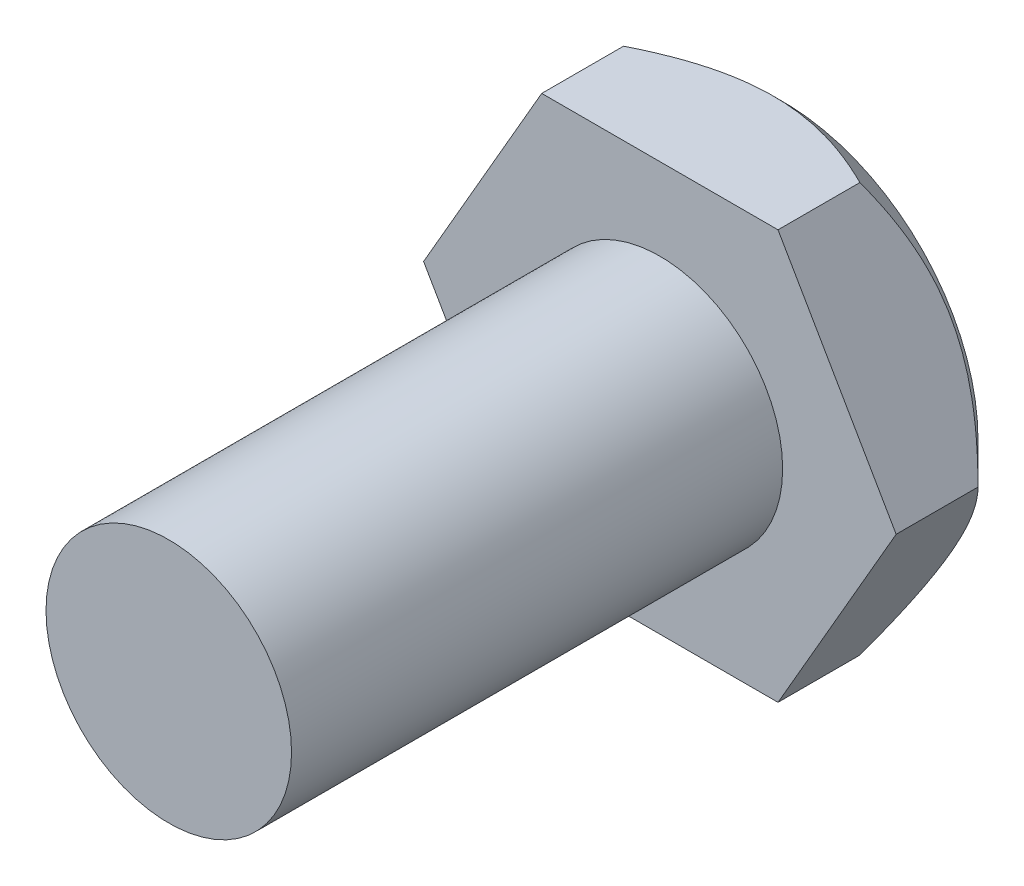
ISO-10303-21;
HEADER;
FILE_DESCRIPTION(('STEP AP214'),'2;1');
FILE_NAME('part.step','',(''),(''),'','','');
FILE_SCHEMA(('AUTOMOTIVE_DESIGN { 1 0 10303 214 1 1 1 1 }'));
ENDSEC;
DATA;
#1=APPLICATION_CONTEXT('core data for automotive mechanical design processes');
#2=APPLICATION_PROTOCOL_DEFINITION('international standard','automotive_design',2000,#1);
#3=PRODUCT_CONTEXT('',#1,'mechanical');
#4=PRODUCT('Part','Part','',(#3));
#5=PRODUCT_RELATED_PRODUCT_CATEGORY('part','',(#4));
#6=PRODUCT_DEFINITION_FORMATION('','',#4);
#7=PRODUCT_DEFINITION_CONTEXT('part definition',#1,'design');
#8=PRODUCT_DEFINITION('design','',#6,#7);
#9=PRODUCT_DEFINITION_SHAPE('','',#8);
#10=(LENGTH_UNIT() NAMED_UNIT(*) SI_UNIT(.MILLI.,.METRE.));
#11=(NAMED_UNIT(*) PLANE_ANGLE_UNIT() SI_UNIT($,.RADIAN.));
#12=(NAMED_UNIT(*) SI_UNIT($,.STERADIAN.) SOLID_ANGLE_UNIT());
#13=UNCERTAINTY_MEASURE_WITH_UNIT(LENGTH_MEASURE(1.E-05),#10,'distance_accuracy_value','');
#14=(GEOMETRIC_REPRESENTATION_CONTEXT(3) GLOBAL_UNCERTAINTY_ASSIGNED_CONTEXT((#13)) GLOBAL_UNIT_ASSIGNED_CONTEXT((#10,
#11,#12)) REPRESENTATION_CONTEXT('',''));
#15=CARTESIAN_POINT('',(0.,0.,0.));
#16=DIRECTION('',(0.,0.,1.));
#17=DIRECTION('',(1.,0.,0.));
#18=AXIS2_PLACEMENT_3D('',#15,#16,#17);
#19=CARTESIAN_POINT('',(2.88675134594813,5.,3.));
#20=DIRECTION('',(0.,-1.,0.));
#21=DIRECTION('',(1.,0.,0.));
#22=AXIS2_PLACEMENT_3D('',#19,#20,#21);
#23=PLANE('',#22);
#24=DIRECTION('',(0.,0.,-1.));
#25=VECTOR('',#24,1.);
#26=CARTESIAN_POINT('',(2.88675134594813,5.,3.));
#27=LINE('',#26,#25);
#28=CARTESIAN_POINT('',(2.88675134594813,5.,3.));
#29=VERTEX_POINT('',#28);
#30=CARTESIAN_POINT('',(2.88675134594813,5.,1.));
#31=VERTEX_POINT('',#30);
#32=EDGE_CURVE('E127',#29,#31,#27,.T.);
#33=ORIENTED_EDGE('',*,*,#32,.T.);
#34=CARTESIAN_POINT('',(8.74641662303044,5.,5.3012084078635));
#35=CARTESIAN_POINT('',(8.61716722747172,5.,5.18900265269319));
#36=CARTESIAN_POINT('',(8.4876177762151,5.,5.07714279282808));
#37=CARTESIAN_POINT('',(8.22783886568772,5.,4.85421137306159));
#38=CARTESIAN_POINT('',(8.09760939532866,5.,4.74313982608443));
#39=CARTESIAN_POINT('',(7.70566734866916,5.,4.41115617610394));
#40=CARTESIAN_POINT('',(7.44281985997347,5.,4.19157843738418));
#41=CARTESIAN_POINT('',(6.90728256215139,5.,3.7521402100456));
#42=CARTESIAN_POINT('',(6.63450482165784,5.,3.53238666470399));
#43=CARTESIAN_POINT('',(6.08382967998017,5.,3.09948407125659));
#44=CARTESIAN_POINT('',(5.80593357662144,5.,2.88633338469646));
#45=CARTESIAN_POINT('',(5.3837875337603,5.,2.57335417688984));
#46=CARTESIAN_POINT('',(5.24208933175031,5.,2.47008359846253));
#47=CARTESIAN_POINT('',(4.95671624927878,5.,2.26631520865752));
#48=CARTESIAN_POINT('',(4.81304144911575,5.,2.16581728513737));
#49=CARTESIAN_POINT('',(4.52327399537158,5.,1.96806860455868));
#50=CARTESIAN_POINT('',(4.37717923691741,5.,1.87082092322893));
#51=CARTESIAN_POINT('',(4.0823598208779,5.,1.68041025635649));
#52=CARTESIAN_POINT('',(3.93363539364329,5.,1.58724691550163));
#53=CARTESIAN_POINT('',(3.63427030631384,5.,1.40660875248023));
#54=CARTESIAN_POINT('',(3.48365224734242,5.,1.31909664823553));
#55=CARTESIAN_POINT('',(3.17899028727331,5.,1.15017049908503));
#56=CARTESIAN_POINT('',(3.02494597608888,5.,1.06875718929084));
#57=CARTESIAN_POINT('',(2.71327651039527,5.,0.913643190475421));
#58=CARTESIAN_POINT('',(2.55565698972105,5.,0.839931271085105));
#59=CARTESIAN_POINT('',(2.23636855072567,5.,0.701954577855007));
#60=CARTESIAN_POINT('',(2.07470123003838,5.,0.637686143454928));
#61=CARTESIAN_POINT('',(1.74341514966671,5.,0.519419891787041));
#62=CARTESIAN_POINT('',(1.57369908899825,5.,0.465690806004495));
#63=CARTESIAN_POINT('',(1.23024809831037,5.,0.372972773426489));
#64=CARTESIAN_POINT('',(1.0565138138452,5.,0.333981476125328));
#65=CARTESIAN_POINT('',(0.707111716198468,5.,0.273340953601918));
#66=CARTESIAN_POINT('',(0.531462959939969,5.,0.251584101926993));
#67=CARTESIAN_POINT('',(0.178842057305417,5.,0.22660543562738));
#68=CARTESIAN_POINT('',(0.00187005969020588,5.,0.22338156795711));
#69=CARTESIAN_POINT('',(-0.351677312644675,5.,0.235729427957372));
#70=CARTESIAN_POINT('',(-0.528251644969158,5.,0.251330345354414));
#71=CARTESIAN_POINT('',(-0.878922878802967,5.,0.300185950940667));
#72=CARTESIAN_POINT('',(-1.05301927886708,5.,0.333444161614109));
#73=CARTESIAN_POINT('',(-1.39870451047178,5.,0.415712242024421));
#74=CARTESIAN_POINT('',(-1.57026635442505,5.,0.464833519014821));
#75=CARTESIAN_POINT('',(-1.90902834046006,5.,0.576149176266492));
#76=CARTESIAN_POINT('',(-2.07622841650064,5.,0.638343754340544));
#77=CARTESIAN_POINT('',(-2.44237261212096,5.,0.788103153381532));
#78=CARTESIAN_POINT('',(-2.64025507818804,5.,0.878241389720331));
#79=CARTESIAN_POINT('',(-3.03013540194518,5.,1.07054933532847));
#80=CARTESIAN_POINT('',(-3.22212979396398,5.,1.17272596527721));
#81=CARTESIAN_POINT('',(-3.60131488951699,5.,1.38644051823751));
#82=CARTESIAN_POINT('',(-3.78849486749643,5.,1.49799731621713));
#83=CARTESIAN_POINT('',(-4.15840113964421,5.,1.72813928385285));
#84=CARTESIAN_POINT('',(-4.34112830476994,5.,1.84672306322436));
#85=CARTESIAN_POINT('',(-4.70385374189567,5.,2.09002844075627));
#86=CARTESIAN_POINT('',(-4.88383213902463,5.,2.21477952902243));
#87=CARTESIAN_POINT('',(-5.24067161838558,5.,2.46866048898819));
#88=CARTESIAN_POINT('',(-5.41753258816022,5.,2.59779051816339));
#89=CARTESIAN_POINT('',(-5.76843263526273,5.,2.85939744264288));
#90=CARTESIAN_POINT('',(-5.94247477144878,5.,2.99187024633416));
#91=CARTESIAN_POINT('',(-6.28836717451651,5.,3.25965261483997));
#92=CARTESIAN_POINT('',(-6.46021736942797,5.,3.39496227241612));
#93=CARTESIAN_POINT('',(-6.81175541238502,5.,3.67565032556453));
#94=CARTESIAN_POINT('',(-6.99133474536111,5.,3.82116441788729));
#95=CARTESIAN_POINT('',(-7.34874142921773,5.,4.11432958177972));
#96=CARTESIAN_POINT('',(-7.52656875943086,5.,4.26198067850785));
#97=CARTESIAN_POINT('',(-7.87878816127491,5.,4.55742406898618));
#98=CARTESIAN_POINT('',(-8.0531965095585,5.,4.70519698599776));
#99=CARTESIAN_POINT('',(-8.40071799614823,5.,5.00218161213357));
#100=CARTESIAN_POINT('',(-8.57383141139475,5.,5.15139299703373));
#101=CARTESIAN_POINT('',(-8.74641662303045,5.,5.3012084078635));
#102=B_SPLINE_CURVE_WITH_KNOTS('',3,(#34,#35,#36,#37,#38,#39,#40,#41,#42,#43,#44,#45,#46,#47,
#48,#49,#50,#51,#52,#53,#54,#55,#56,#57,#58,#59,#60,#61,#62,#63,#64,#65,#66,#67,#68,#69,#70,#71,
#72,#73,#74,#75,#76,#77,#78,#79,#80,#81,#82,#83,#84,#85,#86,#87,#88,#89,#90,#91,#92,#93,#94,#95,
#96,#97,#98,#99,#100,#101),.UNSPECIFIED.,.F.,.F.,(4,2,2,2,2,2,2,2,2,2,2,2,2,2,2,2,2,2,2,2,2,2,2,
2,2,2,2,2,2,2,2,2,2,4),(0.,0.513476804360356,1.02696200771218,2.05440464274526,3.10519307167232,
4.15571863124174,4.68170485901197,5.20766978152951,5.73411909352896,6.26052251646935,
6.78299524430338,7.30553084683204,7.82729351501781,8.34885339673759,8.88235034246745,
9.41576216570623,9.94581605965256,10.4758112341947,11.0066292768165,11.5375532530671,
12.0722901283653,12.6070350953768,13.2588184936859,13.9109784370995,14.5644836027157,
15.2178599015943,15.8747380640423,16.5316398742658,17.1877732869579,17.8439281879699,
18.5373113067271,19.2307025951713,19.9164752192631,20.6020967282287),.UNSPECIFIED.);
#103=CARTESIAN_POINT('',(-2.88675134594813,5.,1.));
#104=VERTEX_POINT('',#103);
#105=EDGE_CURVE('E56',#31,#104,#102,.T.);
#106=ORIENTED_EDGE('',*,*,#105,.T.);
#107=DIRECTION('',(0.,0.,-1.));
#108=VECTOR('',#107,1.);
#109=CARTESIAN_POINT('',(-2.88675134594813,5.,3.));
#110=LINE('',#109,#108);
#111=CARTESIAN_POINT('',(-2.88675134594813,5.,3.));
#112=VERTEX_POINT('',#111);
#113=EDGE_CURVE('E50',#112,#104,#110,.T.);
#114=ORIENTED_EDGE('',*,*,#113,.F.);
#115=DIRECTION('',(-1.,0.,0.));
#116=VECTOR('',#115,1.);
#117=CARTESIAN_POINT('',(2.88675134594813,5.,3.));
#118=LINE('',#117,#116);
#119=EDGE_CURVE('E137',#29,#112,#118,.T.);
#120=ORIENTED_EDGE('',*,*,#119,.F.);
#121=EDGE_LOOP('',(#33,#106,#114,#120));
#122=FACE_BOUND('',#121,.T.);
#123=ADVANCED_FACE('F43',(#122),#23,.F.);
#124=CARTESIAN_POINT('',(-2.88675134594813,5.,3.));
#125=DIRECTION('',(0.866025403784439,-0.5,0.));
#126=DIRECTION('',(0.5,0.866025403784439,0.));
#127=AXIS2_PLACEMENT_3D('',#124,#125,#126);
#128=PLANE('',#127);
#129=ORIENTED_EDGE('',*,*,#113,.T.);
#130=CARTESIAN_POINT('',(-2.88663587589429,5.0002,1.00011547351787));
#131=CARTESIAN_POINT('',(-2.93627227674213,4.91422723182669,0.950483545604261));
#132=CARTESIAN_POINT('',(-2.98629020977268,4.82759363052819,0.902374725286905));
#133=CARTESIAN_POINT('',(-3.08716399407135,4.65287511097116,0.809666631329779));
#134=CARTESIAN_POINT('',(-3.13802028490869,4.56478943135639,0.765069274501487));
#135=CARTESIAN_POINT('',(-3.29243146040539,4.29734143013967,0.636859072128257));
#136=CARTESIAN_POINT('',(-3.39729352840467,4.11571500057817,0.559375065501523));
#137=CARTESIAN_POINT('',(-3.60875628789733,3.74945075722817,0.42668894442552));
#138=CARTESIAN_POINT('',(-3.71530292847297,3.56490656237538,0.371152540645841));
#139=CARTESIAN_POINT('',(-3.87687459445693,3.28505622782761,0.306910494047523));
#140=CARTESIAN_POINT('',(-3.93096969797871,3.19136076008719,0.288682163338643));
#141=CARTESIAN_POINT('',(-4.03961794604879,3.00317647427646,0.258992187126128));
#142=CARTESIAN_POINT('',(-4.09417102090354,2.90868777691894,0.247529530305092));
#143=CARTESIAN_POINT('',(-4.22710825098567,2.67843374019921,0.228310861745989));
#144=CARTESIAN_POINT('',(-4.30563563855842,2.54242031513756,0.224278288259721));
#145=CARTESIAN_POINT('',(-4.46254889182114,2.27063858810559,0.231045854105319));
#146=CARTESIAN_POINT('',(-4.54093469825831,2.13487038876416,0.241851192971007));
#147=CARTESIAN_POINT('',(-4.69696731557989,1.86461396792522,0.27765764989805));
#148=CARTESIAN_POINT('',(-4.77461320108937,1.73012734922414,0.302674643958276));
#149=CARTESIAN_POINT('',(-4.92857043343806,1.46346560060351,0.36554432498945));
#150=CARTESIAN_POINT('',(-5.00488188213305,1.3312902942646,0.403396027767576));
#151=CARTESIAN_POINT('',(-5.14035048372464,1.09665179347766,0.481269886760554));
#152=CARTESIAN_POINT('',(-5.1998075641558,0.993669109301183,0.519244250419034));
#153=CARTESIAN_POINT('',(-5.31765436322279,0.789552465807812,0.60131262617396));
#154=CARTESIAN_POINT('',(-5.37604404938545,0.688418562736066,0.645406824103566));
#155=CARTESIAN_POINT('',(-5.49157215635532,0.488318011762015,0.73872638535237));
#156=CARTESIAN_POINT('',(-5.54871386288991,0.389345672812901,0.787935612709399));
#157=CARTESIAN_POINT('',(-5.66193913120708,0.193233755386953,0.890839122843011));
#158=CARTESIAN_POINT('',(-5.7180233165161,0.0960930969306156,0.944530654549024));
#159=CARTESIAN_POINT('',(-5.7736181619501,-0.00020000000000107,1.00011547351787));
#160=B_SPLINE_CURVE_WITH_KNOTS('',3,(#130,#131,#132,#133,#134,#135,#136,#137,#138,#139,#140,
#141,#142,#143,#144,#145,#146,#147,#148,#149,#150,#151,#152,#153,#154,#155,#156,#157,#158,#159),
.UNSPECIFIED.,.F.,.F.,(4,2,2,2,2,2,2,2,2,2,2,2,2,2,4),(0.,0.33294561620957,0.666071736106994,
1.33592065243335,1.99513262597482,2.32409207808825,2.65300234563692,3.12358963991985,
3.59434188052355,4.06562104077029,4.53686407049613,4.91117956742319,5.28550643319671,
5.65868635377115,6.03163889109472),.UNSPECIFIED.);
#161=CARTESIAN_POINT('',(-5.77350269189626,0.,1.));
#162=VERTEX_POINT('',#161);
#163=EDGE_CURVE('E100',#104,#162,#160,.T.);
#164=ORIENTED_EDGE('',*,*,#163,.T.);
#165=DIRECTION('',(0.,0.,-1.));
#166=VECTOR('',#165,1.);
#167=CARTESIAN_POINT('',(-5.77350269189626,0.,3.));
#168=LINE('',#167,#166);
#169=CARTESIAN_POINT('',(-5.77350269189626,0.,3.));
#170=VERTEX_POINT('',#169);
#171=EDGE_CURVE('E111',#170,#162,#168,.T.);
#172=ORIENTED_EDGE('',*,*,#171,.F.);
#173=DIRECTION('',(-0.5,-0.866025403784439,0.));
#174=VECTOR('',#173,1.);
#175=CARTESIAN_POINT('',(-2.88675134594813,5.,3.));
#176=LINE('',#175,#174);
#177=EDGE_CURVE('E135',#112,#170,#176,.T.);
#178=ORIENTED_EDGE('',*,*,#177,.F.);
#179=EDGE_LOOP('',(#129,#164,#172,#178));
#180=FACE_BOUND('',#179,.T.);
#181=ADVANCED_FACE('F109',(#180),#128,.F.);
#182=CARTESIAN_POINT('',(-5.77350269189626,0.,3.));
#183=DIRECTION('',(0.866025403784439,0.5,0.));
#184=DIRECTION('',(-0.5,0.866025403784439,0.));
#185=AXIS2_PLACEMENT_3D('',#182,#183,#184);
#186=PLANE('',#185);
#187=ORIENTED_EDGE('',*,*,#171,.T.);
#188=CARTESIAN_POINT('',(-5.7736181619501,0.000199999999999427,1.00011547351787));
#189=CARTESIAN_POINT('',(-5.72398176110226,-0.0857727681733085,0.950483545604261));
#190=CARTESIAN_POINT('',(-5.6739638280717,-0.172406369471811,0.902374725286906));
#191=CARTESIAN_POINT('',(-5.57309004377304,-0.347124889028842,0.80966663132978));
#192=CARTESIAN_POINT('',(-5.5222337529357,-0.435210568643613,0.765069274501488));
#193=CARTESIAN_POINT('',(-5.367822577439,-0.702658569860335,0.636859072128257));
#194=CARTESIAN_POINT('',(-5.26296050943971,-0.884284999421835,0.559375065501522));
#195=CARTESIAN_POINT('',(-5.05149774994706,-1.25054924277183,0.42668894442552));
#196=CARTESIAN_POINT('',(-4.94495110937142,-1.43509343762462,0.371152540645841));
#197=CARTESIAN_POINT('',(-4.78337944338746,-1.71494377217239,0.306910494047522));
#198=CARTESIAN_POINT('',(-4.72928433986568,-1.80863923991281,0.288682163338643));
#199=CARTESIAN_POINT('',(-4.62063609179559,-1.99682352572355,0.258992187126128));
#200=CARTESIAN_POINT('',(-4.56608301694085,-2.09131222308107,0.247529530305092));
#201=CARTESIAN_POINT('',(-4.43314578685872,-2.32156625980079,0.228310861745989));
#202=CARTESIAN_POINT('',(-4.35461839928597,-2.45757968486244,0.22427828825972));
#203=CARTESIAN_POINT('',(-4.19770514602324,-2.72936141189441,0.231045854105318));
#204=CARTESIAN_POINT('',(-4.11931933958608,-2.86512961123584,0.241851192971006));
#205=CARTESIAN_POINT('',(-3.96328672226449,-3.13538603207478,0.277657649898049));
#206=CARTESIAN_POINT('',(-3.88564083675502,-3.26987265077586,0.302674643958275));
#207=CARTESIAN_POINT('',(-3.73168360440632,-3.53653439939649,0.365544324989449));
#208=CARTESIAN_POINT('',(-3.65537215571133,-3.6687097057354,0.403396027767576));
#209=CARTESIAN_POINT('',(-3.51990355411974,-3.90334820652234,0.481269886760554));
#210=CARTESIAN_POINT('',(-3.46044647368858,-4.00633089069882,0.519244250419033));
#211=CARTESIAN_POINT('',(-3.3425996746216,-4.21044753419219,0.60131262617396));
#212=CARTESIAN_POINT('',(-3.28420998845893,-4.31158143726393,0.645406824103565));
#213=CARTESIAN_POINT('',(-3.16868188148907,-4.51168198823799,0.73872638535237));
#214=CARTESIAN_POINT('',(-3.11154017495447,-4.6106543271871,0.787935612709399));
#215=CARTESIAN_POINT('',(-2.99831490663731,-4.80676624461305,0.890839122843011));
#216=CARTESIAN_POINT('',(-2.94223072132828,-4.90390690306939,0.944530654549024));
#217=CARTESIAN_POINT('',(-2.88663587589429,-5.0002,1.00011547351787));
#218=B_SPLINE_CURVE_WITH_KNOTS('',3,(#188,#189,#190,#191,#192,#193,#194,#195,#196,#197,#198,
#199,#200,#201,#202,#203,#204,#205,#206,#207,#208,#209,#210,#211,#212,#213,#214,#215,#216,#217),
.UNSPECIFIED.,.F.,.F.,(4,2,2,2,2,2,2,2,2,2,2,2,2,2,4),(0.,0.332945616209569,0.666071736106994,
1.33592065243335,1.99513262597482,2.32409207808825,2.65300234563692,3.12358963991985,
3.59434188052356,4.06562104077029,4.53686407049613,4.91117956742319,5.28550643319671,
5.65868635377115,6.03163889109472),.UNSPECIFIED.);
#219=CARTESIAN_POINT('',(-2.88675134594813,-5.,1.));
#220=VERTEX_POINT('',#219);
#221=EDGE_CURVE('E98',#162,#220,#218,.T.);
#222=ORIENTED_EDGE('',*,*,#221,.T.);
#223=DIRECTION('',(0.,0.,-1.));
#224=VECTOR('',#223,1.);
#225=CARTESIAN_POINT('',(-2.88675134594813,-5.,3.));
#226=LINE('',#225,#224);
#227=CARTESIAN_POINT('',(-2.88675134594813,-5.,3.));
#228=VERTEX_POINT('',#227);
#229=EDGE_CURVE('E120',#228,#220,#226,.T.);
#230=ORIENTED_EDGE('',*,*,#229,.F.);
#231=DIRECTION('',(0.5,-0.866025403784438,0.));
#232=VECTOR('',#231,1.);
#233=CARTESIAN_POINT('',(-5.77350269189626,0.,3.));
#234=LINE('',#233,#232);
#235=EDGE_CURVE('E116',#170,#228,#234,.T.);
#236=ORIENTED_EDGE('',*,*,#235,.F.);
#237=EDGE_LOOP('',(#187,#222,#230,#236));
#238=FACE_BOUND('',#237,.T.);
#239=ADVANCED_FACE('F114',(#238),#186,.F.);
#240=CARTESIAN_POINT('',(-2.88675134594813,-5.,3.));
#241=DIRECTION('',(0.,1.,0.));
#242=DIRECTION('',(-1.,0.,0.));
#243=AXIS2_PLACEMENT_3D('',#240,#241,#242);
#244=PLANE('',#243);
#245=ORIENTED_EDGE('',*,*,#229,.T.);
#246=CARTESIAN_POINT('',(-8.74641662303044,-5.,5.3012084078635));
#247=CARTESIAN_POINT('',(-8.61716722747172,-5.,5.18900265269319));
#248=CARTESIAN_POINT('',(-8.4876177762151,-5.,5.07714279282808));
#249=CARTESIAN_POINT('',(-8.22783886568772,-5.,4.85421137306158));
#250=CARTESIAN_POINT('',(-8.09760939532866,-5.,4.74313982608443));
#251=CARTESIAN_POINT('',(-7.70566734866915,-5.,4.41115617610394));
#252=CARTESIAN_POINT('',(-7.44281985997347,-5.,4.19157843738418));
#253=CARTESIAN_POINT('',(-6.90728256215139,-5.,3.7521402100456));
#254=CARTESIAN_POINT('',(-6.63450482165784,-5.,3.53238666470399));
#255=CARTESIAN_POINT('',(-6.08382967998017,-5.,3.09948407125659));
#256=CARTESIAN_POINT('',(-5.80593357662143,-5.,2.88633338469646));
#257=CARTESIAN_POINT('',(-5.3837875337603,-5.,2.57335417688984));
#258=CARTESIAN_POINT('',(-5.24208933175031,-5.,2.47008359846253));
#259=CARTESIAN_POINT('',(-4.95671624927878,-5.,2.26631520865752));
#260=CARTESIAN_POINT('',(-4.81304144911575,-5.,2.16581728513737));
#261=CARTESIAN_POINT('',(-4.52327399537158,-5.,1.96806860455868));
#262=CARTESIAN_POINT('',(-4.37717923691741,-5.,1.87082092322893));
#263=CARTESIAN_POINT('',(-4.0823598208779,-5.,1.68041025635649));
#264=CARTESIAN_POINT('',(-3.93363539364329,-5.,1.58724691550163));
#265=CARTESIAN_POINT('',(-3.63427030631384,-5.,1.40660875248022));
#266=CARTESIAN_POINT('',(-3.48365224734242,-5.,1.31909664823553));
#267=CARTESIAN_POINT('',(-3.17899028727331,-5.,1.15017049908503));
#268=CARTESIAN_POINT('',(-3.02494597608888,-5.,1.06875718929084));
#269=CARTESIAN_POINT('',(-2.71327651039527,-5.,0.91364319047542));
#270=CARTESIAN_POINT('',(-2.55565698972105,-5.,0.839931271085105));
#271=CARTESIAN_POINT('',(-2.23636855072567,-5.,0.701954577855007));
#272=CARTESIAN_POINT('',(-2.07470123003838,-5.,0.637686143454927));
#273=CARTESIAN_POINT('',(-1.74341514966671,-5.,0.519419891787041));
#274=CARTESIAN_POINT('',(-1.57369908899825,-5.,0.465690806004495));
#275=CARTESIAN_POINT('',(-1.23024809831037,-5.,0.37297277342649));
#276=CARTESIAN_POINT('',(-1.0565138138452,-5.,0.333981476125329));
#277=CARTESIAN_POINT('',(-0.707111716198468,-5.,0.273340953601918));
#278=CARTESIAN_POINT('',(-0.531462959939969,-5.,0.251584101926994));
#279=CARTESIAN_POINT('',(-0.178842057305416,-5.,0.226605435627381));
#280=CARTESIAN_POINT('',(-0.00187005969020575,-5.,0.22338156795711));
#281=CARTESIAN_POINT('',(0.351677312644676,-5.,0.235729427957372));
#282=CARTESIAN_POINT('',(0.528251644969159,-5.,0.251330345354415));
#283=CARTESIAN_POINT('',(0.878922878802968,-5.,0.300185950940667));
#284=CARTESIAN_POINT('',(1.05301927886708,-5.,0.33344416161411));
#285=CARTESIAN_POINT('',(1.39870451047178,-5.,0.415712242024421));
#286=CARTESIAN_POINT('',(1.57026635442505,-5.,0.464833519014821));
#287=CARTESIAN_POINT('',(1.90902834046006,-5.,0.576149176266492));
#288=CARTESIAN_POINT('',(2.07622841650064,-5.,0.638343754340544));
#289=CARTESIAN_POINT('',(2.44237261212096,-5.,0.788103153381532));
#290=CARTESIAN_POINT('',(2.64025507818804,-5.,0.878241389720331));
#291=CARTESIAN_POINT('',(3.03013540194518,-5.,1.07054933532847));
#292=CARTESIAN_POINT('',(3.22212979396398,-5.,1.1727259652772));
#293=CARTESIAN_POINT('',(3.60131488951699,-5.,1.38644051823751));
#294=CARTESIAN_POINT('',(3.78849486749642,-5.,1.49799731621713));
#295=CARTESIAN_POINT('',(4.15840113964421,-5.,1.72813928385285));
#296=CARTESIAN_POINT('',(4.34112830476994,-5.,1.84672306322436));
#297=CARTESIAN_POINT('',(4.70385374189567,-5.,2.09002844075627));
#298=CARTESIAN_POINT('',(4.88383213902462,-5.,2.21477952902243));
#299=CARTESIAN_POINT('',(5.24067161838558,-5.,2.46866048898819));
#300=CARTESIAN_POINT('',(5.41753258816022,-5.,2.59779051816339));
#301=CARTESIAN_POINT('',(5.76843263526273,-5.,2.85939744264287));
#302=CARTESIAN_POINT('',(5.94247477144877,-5.,2.99187024633416));
#303=CARTESIAN_POINT('',(6.2883671745165,-5.,3.25965261483996));
#304=CARTESIAN_POINT('',(6.46021736942796,-5.,3.39496227241611));
#305=CARTESIAN_POINT('',(6.81175541238501,-5.,3.67565032556453));
#306=CARTESIAN_POINT('',(6.9913347453611,-5.,3.82116441788729));
#307=CARTESIAN_POINT('',(7.34874142921773,-5.,4.11432958177972));
#308=CARTESIAN_POINT('',(7.52656875943086,-5.,4.26198067850785));
#309=CARTESIAN_POINT('',(7.87878816127491,-5.,4.55742406898618));
#310=CARTESIAN_POINT('',(8.0531965095585,-5.,4.70519698599776));
#311=CARTESIAN_POINT('',(8.40071799614823,-5.,5.00218161213357));
#312=CARTESIAN_POINT('',(8.57383141139475,-5.,5.15139299703373));
#313=CARTESIAN_POINT('',(8.74641662303045,-5.,5.3012084078635));
#314=B_SPLINE_CURVE_WITH_KNOTS('',3,(#246,#247,#248,#249,#250,#251,#252,#253,#254,#255,#256,
#257,#258,#259,#260,#261,#262,#263,#264,#265,#266,#267,#268,#269,#270,#271,#272,#273,#274,#275,
#276,#277,#278,#279,#280,#281,#282,#283,#284,#285,#286,#287,#288,#289,#290,#291,#292,#293,#294,
#295,#296,#297,#298,#299,#300,#301,#302,#303,#304,#305,#306,#307,#308,#309,#310,#311,#312,#313),
.UNSPECIFIED.,.F.,.F.,(4,2,2,2,2,2,2,2,2,2,2,2,2,2,2,2,2,2,2,2,2,2,2,2,2,2,2,2,2,2,2,2,2,4),(0.,
0.513476804360357,1.02696200771218,2.05440464274526,3.10519307167232,4.15571863124174,
4.68170485901197,5.2076697815295,5.73411909352896,6.26052251646935,6.78299524430337,
7.30553084683203,7.82729351501781,8.34885339673758,8.88235034246745,9.41576216570623,
9.94581605965256,10.4758112341947,11.0066292768165,11.5375532530671,12.0722901283653,
12.6070350953768,13.2588184936859,13.9109784370995,14.5644836027157,15.2178599015943,
15.8747380640423,16.5316398742658,17.1877732869579,17.8439281879698,18.5373113067271,
19.2307025951713,19.9164752192631,20.6020967282287),.UNSPECIFIED.);
#315=CARTESIAN_POINT('',(2.88675134594813,-5.,1.));
#316=VERTEX_POINT('',#315);
#317=EDGE_CURVE('E103',#220,#316,#314,.T.);
#318=ORIENTED_EDGE('',*,*,#317,.T.);
#319=DIRECTION('',(0.,0.,-1.));
#320=VECTOR('',#319,1.);
#321=CARTESIAN_POINT('',(2.88675134594813,-5.,3.));
#322=LINE('',#321,#320);
#323=CARTESIAN_POINT('',(2.88675134594813,-5.,3.));
#324=VERTEX_POINT('',#323);
#325=EDGE_CURVE('E117',#324,#316,#322,.T.);
#326=ORIENTED_EDGE('',*,*,#325,.F.);
#327=DIRECTION('',(1.,0.,0.));
#328=VECTOR('',#327,1.);
#329=CARTESIAN_POINT('',(-2.88675134594813,-5.,3.));
#330=LINE('',#329,#328);
#331=EDGE_CURVE('E132',#228,#324,#330,.T.);
#332=ORIENTED_EDGE('',*,*,#331,.F.);
#333=EDGE_LOOP('',(#245,#318,#326,#332));
#334=FACE_BOUND('',#333,.T.);
#335=ADVANCED_FACE('F192',(#334),#244,.F.);
#336=CARTESIAN_POINT('',(2.88675134594813,-5.,3.));
#337=DIRECTION('',(-0.866025403784439,0.5,0.));
#338=DIRECTION('',(-0.5,-0.866025403784439,0.));
#339=AXIS2_PLACEMENT_3D('',#336,#337,#338);
#340=PLANE('',#339);
#341=ORIENTED_EDGE('',*,*,#325,.T.);
#342=CARTESIAN_POINT('',(2.88663587589429,-5.0002,1.00011547351787));
#343=CARTESIAN_POINT('',(2.93627227674213,-4.91422723182669,0.950483545604261));
#344=CARTESIAN_POINT('',(2.98629020977269,-4.82759363052819,0.902374725286905));
#345=CARTESIAN_POINT('',(3.08716399407135,-4.65287511097116,0.80966663132978));
#346=CARTESIAN_POINT('',(3.13802028490869,-4.56478943135639,0.765069274501487));
#347=CARTESIAN_POINT('',(3.29243146040539,-4.29734143013967,0.636859072128257));
#348=CARTESIAN_POINT('',(3.39729352840467,-4.11571500057817,0.559375065501523));
#349=CARTESIAN_POINT('',(3.60875628789733,-3.74945075722817,0.426688944425521));
#350=CARTESIAN_POINT('',(3.71530292847297,-3.56490656237538,0.371152540645842));
#351=CARTESIAN_POINT('',(3.87687459445693,-3.28505622782762,0.306910494047523));
#352=CARTESIAN_POINT('',(3.93096969797871,-3.19136076008719,0.288682163338643));
#353=CARTESIAN_POINT('',(4.03961794604879,-3.00317647427646,0.258992187126128));
#354=CARTESIAN_POINT('',(4.09417102090354,-2.90868777691894,0.247529530305092));
#355=CARTESIAN_POINT('',(4.22710825098567,-2.67843374019921,0.228310861745991));
#356=CARTESIAN_POINT('',(4.30563563855842,-2.54242031513756,0.224278288259722));
#357=CARTESIAN_POINT('',(4.46254889182114,-2.27063858810559,0.23104585410532));
#358=CARTESIAN_POINT('',(4.54093469825831,-2.13487038876416,0.241851192971008));
#359=CARTESIAN_POINT('',(4.69696731557989,-1.86461396792523,0.27765764989805));
#360=CARTESIAN_POINT('',(4.77461320108937,-1.73012734922414,0.302674643958276));
#361=CARTESIAN_POINT('',(4.92857043343806,-1.46346560060351,0.36554432498945));
#362=CARTESIAN_POINT('',(5.00488188213305,-1.33129029426461,0.403396027767577));
#363=CARTESIAN_POINT('',(5.14035048372464,-1.09665179347767,0.481269886760554));
#364=CARTESIAN_POINT('',(5.1998075641558,-0.993669109301185,0.519244250419034));
#365=CARTESIAN_POINT('',(5.31765436322279,-0.789552465807813,0.60131262617396));
#366=CARTESIAN_POINT('',(5.37604404938546,-0.688418562736067,0.645406824103566));
#367=CARTESIAN_POINT('',(5.49157215635532,-0.488318011762016,0.738726385352371));
#368=CARTESIAN_POINT('',(5.54871386288991,-0.389345672812902,0.787935612709401));
#369=CARTESIAN_POINT('',(5.66193913120708,-0.193233755386953,0.890839122843013));
#370=CARTESIAN_POINT('',(5.7180233165161,-0.0960930969306155,0.944530654549025));
#371=CARTESIAN_POINT('',(5.7736181619501,0.000200000000001084,1.00011547351787));
#372=B_SPLINE_CURVE_WITH_KNOTS('',3,(#342,#343,#344,#345,#346,#347,#348,#349,#350,#351,#352,
#353,#354,#355,#356,#357,#358,#359,#360,#361,#362,#363,#364,#365,#366,#367,#368,#369,#370,#371),
.UNSPECIFIED.,.F.,.F.,(4,2,2,2,2,2,2,2,2,2,2,2,2,2,4),(0.,0.33294561620957,0.666071736106994,
1.33592065243335,1.99513262597482,2.32409207808825,2.65300234563692,3.12358963991984,
3.59434188052355,4.06562104077029,4.53686407049613,4.91117956742318,5.28550643319671,
5.65868635377115,6.03163889109472),.UNSPECIFIED.);
#373=CARTESIAN_POINT('',(5.77350269189626,0.,1.));
#374=VERTEX_POINT('',#373);
#375=EDGE_CURVE('E171',#316,#374,#372,.T.);
#376=ORIENTED_EDGE('',*,*,#375,.T.);
#377=DIRECTION('',(0.,0.,-1.));
#378=VECTOR('',#377,1.);
#379=CARTESIAN_POINT('',(5.77350269189626,0.,3.));
#380=LINE('',#379,#378);
#381=CARTESIAN_POINT('',(5.77350269189626,0.,3.));
#382=VERTEX_POINT('',#381);
#383=EDGE_CURVE('E124',#382,#374,#380,.T.);
#384=ORIENTED_EDGE('',*,*,#383,.F.);
#385=DIRECTION('',(0.5,0.866025403784439,0.));
#386=VECTOR('',#385,1.);
#387=CARTESIAN_POINT('',(2.88675134594813,-5.,3.));
#388=LINE('',#387,#386);
#389=EDGE_CURVE('E128',#324,#382,#388,.T.);
#390=ORIENTED_EDGE('',*,*,#389,.F.);
#391=EDGE_LOOP('',(#341,#376,#384,#390));
#392=FACE_BOUND('',#391,.T.);
#393=ADVANCED_FACE('F218',(#392),#340,.F.);
#394=CARTESIAN_POINT('',(5.77350269189626,0.,3.));
#395=DIRECTION('',(-0.866025403784438,-0.5,0.));
#396=DIRECTION('',(0.5,-0.866025403784439,0.));
#397=AXIS2_PLACEMENT_3D('',#394,#395,#396);
#398=PLANE('',#397);
#399=ORIENTED_EDGE('',*,*,#383,.T.);
#400=CARTESIAN_POINT('',(5.7736181619501,-0.000199999999999145,1.00011547351787));
#401=CARTESIAN_POINT('',(5.72398176110226,0.085772768173309,0.950483545604262));
#402=CARTESIAN_POINT('',(5.6739638280717,0.172406369471811,0.902374725286906));
#403=CARTESIAN_POINT('',(5.57309004377304,0.347124889028842,0.809666631329781));
#404=CARTESIAN_POINT('',(5.5222337529357,0.435210568643614,0.765069274501489));
#405=CARTESIAN_POINT('',(5.367822577439,0.702658569860335,0.636859072128258));
#406=CARTESIAN_POINT('',(5.26296050943971,0.884284999421835,0.559375065501523));
#407=CARTESIAN_POINT('',(5.05149774994706,1.25054924277183,0.426688944425521));
#408=CARTESIAN_POINT('',(4.94495110937142,1.43509343762462,0.371152540645843));
#409=CARTESIAN_POINT('',(4.78337944338746,1.71494377217239,0.306910494047524));
#410=CARTESIAN_POINT('',(4.72928433986568,1.80863923991281,0.288682163338643));
#411=CARTESIAN_POINT('',(4.62063609179559,1.99682352572354,0.258992187126128));
#412=CARTESIAN_POINT('',(4.56608301694085,2.09131222308107,0.247529530305092));
#413=CARTESIAN_POINT('',(4.43314578685872,2.32156625980079,0.228310861745991));
#414=CARTESIAN_POINT('',(4.35461839928597,2.45757968486244,0.224278288259722));
#415=CARTESIAN_POINT('',(4.19770514602324,2.72936141189441,0.23104585410532));
#416=CARTESIAN_POINT('',(4.11931933958608,2.86512961123584,0.241851192971008));
#417=CARTESIAN_POINT('',(3.96328672226449,3.13538603207478,0.27765764989805));
#418=CARTESIAN_POINT('',(3.88564083675502,3.26987265077586,0.302674643958277));
#419=CARTESIAN_POINT('',(3.73168360440633,3.53653439939649,0.365544324989451));
#420=CARTESIAN_POINT('',(3.65537215571134,3.66870970573539,0.403396027767577));
#421=CARTESIAN_POINT('',(3.51990355411975,3.90334820652234,0.481269886760554));
#422=CARTESIAN_POINT('',(3.46044647368858,4.00633089069882,0.519244250419034));
#423=CARTESIAN_POINT('',(3.3425996746216,4.21044753419219,0.601312626173961));
#424=CARTESIAN_POINT('',(3.28420998845893,4.31158143726393,0.645406824103566));
#425=CARTESIAN_POINT('',(3.16868188148907,4.51168198823799,0.73872638535237));
#426=CARTESIAN_POINT('',(3.11154017495447,4.6106543271871,0.787935612709399));
#427=CARTESIAN_POINT('',(2.99831490663731,4.80676624461305,0.890839122843011));
#428=CARTESIAN_POINT('',(2.94223072132829,4.90390690306938,0.944530654549024));
#429=CARTESIAN_POINT('',(2.88663587589429,5.0002,1.00011547351787));
#430=B_SPLINE_CURVE_WITH_KNOTS('',3,(#400,#401,#402,#403,#404,#405,#406,#407,#408,#409,#410,
#411,#412,#413,#414,#415,#416,#417,#418,#419,#420,#421,#422,#423,#424,#425,#426,#427,#428,#429),
.UNSPECIFIED.,.F.,.F.,(4,2,2,2,2,2,2,2,2,2,2,2,2,2,4),(0.,0.33294561620957,0.666071736106994,
1.33592065243335,1.99513262597482,2.32409207808825,2.65300234563692,3.12358963991985,
3.59434188052355,4.06562104077029,4.53686407049613,4.91117956742319,5.28550643319671,
5.65868635377115,6.03163889109472),.UNSPECIFIED.);
#431=EDGE_CURVE('E163',#374,#31,#430,.T.);
#432=ORIENTED_EDGE('',*,*,#431,.T.);
#433=ORIENTED_EDGE('',*,*,#32,.F.);
#434=DIRECTION('',(-0.5,0.866025403784439,0.));
#435=VECTOR('',#434,1.);
#436=CARTESIAN_POINT('',(5.77350269189626,0.,3.));
#437=LINE('',#436,#435);
#438=EDGE_CURVE('E67',#382,#29,#437,.T.);
#439=ORIENTED_EDGE('',*,*,#438,.F.);
#440=EDGE_LOOP('',(#399,#432,#433,#439));
#441=FACE_BOUND('',#440,.T.);
#442=ADVANCED_FACE('F203',(#441),#398,.F.);
#443=CARTESIAN_POINT('',(0.,0.,3.));
#444=DIRECTION('',(0.,0.,1.));
#445=DIRECTION('',(1.,0.,0.));
#446=AXIS2_PLACEMENT_3D('',#443,#444,#445);
#447=PLANE('',#446);
#448=CARTESIAN_POINT('',(0.,0.,3.));
#449=DIRECTION('',(0.,0.,1.));
#450=DIRECTION('',(1.,0.,0.));
#451=AXIS2_PLACEMENT_3D('',#448,#449,#450);
#452=CIRCLE('',#451,3.);
#453=CARTESIAN_POINT('',(3.,0.,3.));
#454=VERTEX_POINT('',#453);
#455=EDGE_CURVE('E11',#454,#454,#452,.T.);
#456=ORIENTED_EDGE('',*,*,#455,.F.);
#457=EDGE_LOOP('',(#456));
#458=FACE_BOUND('',#457,.T.);
#459=ORIENTED_EDGE('',*,*,#119,.T.);
#460=ORIENTED_EDGE('',*,*,#177,.T.);
#461=ORIENTED_EDGE('',*,*,#235,.T.);
#462=ORIENTED_EDGE('',*,*,#331,.T.);
#463=ORIENTED_EDGE('',*,*,#389,.T.);
#464=ORIENTED_EDGE('',*,*,#438,.T.);
#465=EDGE_LOOP('',(#459,#460,#461,#462,#463,#464));
#466=FACE_BOUND('',#465,.T.);
#467=ADVANCED_FACE('F216',(#458,#466),#447,.T.);
#468=CARTESIAN_POINT('',(0.,0.,15.));
#469=DIRECTION('',(0.,0.,-1.));
#470=DIRECTION('',(-1.,0.,0.));
#471=AXIS2_PLACEMENT_3D('',#468,#469,#470);
#472=CYLINDRICAL_SURFACE('',#471,3.);
#473=CARTESIAN_POINT('',(0.,0.,15.));
#474=DIRECTION('',(0.,0.,1.));
#475=DIRECTION('',(1.,0.,0.));
#476=AXIS2_PLACEMENT_3D('',#473,#474,#475);
#477=CIRCLE('',#476,3.);
#478=CARTESIAN_POINT('',(3.,0.,15.));
#479=VERTEX_POINT('',#478);
#480=EDGE_CURVE('E139',#479,#479,#477,.T.);
#481=ORIENTED_EDGE('',*,*,#480,.F.);
#482=EDGE_LOOP('',(#481));
#483=FACE_BOUND('',#482,.T.);
#484=ORIENTED_EDGE('',*,*,#455,.T.);
#485=EDGE_LOOP('',(#484));
#486=FACE_BOUND('',#485,.T.);
#487=ADVANCED_FACE('F233',(#483,#486),#472,.T.);
#488=CARTESIAN_POINT('',(0.,0.,15.));
#489=DIRECTION('',(0.,0.,1.));
#490=DIRECTION('',(1.,0.,0.));
#491=AXIS2_PLACEMENT_3D('',#488,#489,#490);
#492=PLANE('',#491);
#493=ORIENTED_EDGE('',*,*,#480,.T.);
#494=EDGE_LOOP('',(#493));
#495=FACE_BOUND('',#494,.T.);
#496=ADVANCED_FACE('F155',(#495),#492,.T.);
#497=CARTESIAN_POINT('',(0.,0.,1.));
#498=DIRECTION('',(0.,0.,1.));
#499=DIRECTION('',(1.,0.,0.));
#500=AXIS2_PLACEMENT_3D('',#497,#498,#499);
#501=CONICAL_SURFACE('',#500,5.77350269189626,0.785398163397453);
#502=CARTESIAN_POINT('',(0.,0.,0.));
#503=DIRECTION('',(0.,0.,-1.));
#504=DIRECTION('',(-1.,0.,0.));
#505=AXIS2_PLACEMENT_3D('',#502,#503,#504);
#506=CIRCLE('',#505,4.77350269189625);
#507=CARTESIAN_POINT('',(-4.77350269189625,0.,0.));
#508=VERTEX_POINT('',#507);
#509=EDGE_CURVE('E210',#508,#508,#506,.T.);
#510=ORIENTED_EDGE('',*,*,#509,.F.);
#511=EDGE_LOOP('',(#510));
#512=FACE_BOUND('',#511,.T.);
#513=ORIENTED_EDGE('',*,*,#431,.F.);
#514=ORIENTED_EDGE('',*,*,#375,.F.);
#515=ORIENTED_EDGE('',*,*,#317,.F.);
#516=ORIENTED_EDGE('',*,*,#221,.F.);
#517=ORIENTED_EDGE('',*,*,#163,.F.);
#518=ORIENTED_EDGE('',*,*,#105,.F.);
#519=EDGE_LOOP('',(#513,#514,#515,#516,#517,#518));
#520=FACE_BOUND('',#519,.T.);
#521=ADVANCED_FACE('F96',(#512,#520),#501,.T.);
#522=CARTESIAN_POINT('',(0.,0.,0.));
#523=DIRECTION('',(0.,0.,1.));
#524=DIRECTION('',(1.,0.,0.));
#525=AXIS2_PLACEMENT_3D('',#522,#523,#524);
#526=PLANE('',#525);
#527=ORIENTED_EDGE('',*,*,#509,.T.);
#528=EDGE_LOOP('',(#527));
#529=FACE_BOUND('',#528,.T.);
#530=ADVANCED_FACE('F153',(#529),#526,.F.);
#531=CLOSED_SHELL('',(#123,#181,#239,#335,#393,#442,#467,#487,#496,#521,#530));
#532=MANIFOLD_SOLID_BREP('B2',#531);
#533=ADVANCED_BREP_SHAPE_REPRESENTATION('',(#18,#532),#14);
#534=SHAPE_DEFINITION_REPRESENTATION(#9,#533);
ENDSEC;
END-ISO-10303-21;
